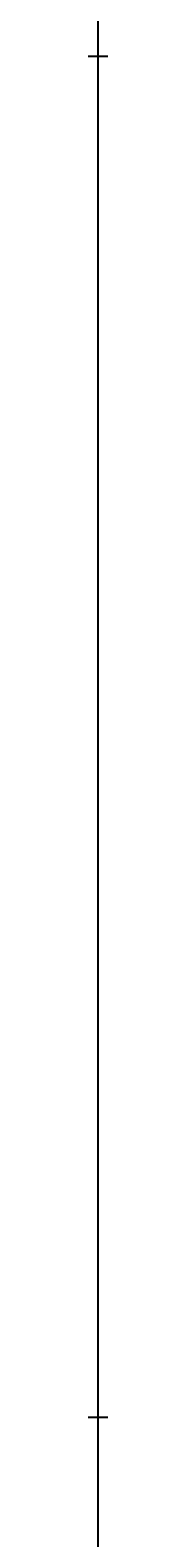
# Model space of a CAD drawing. Units: inches. Extents: x 35362 to 73946, y 43607 to 67532.
# Tile 36 of 134: x 48373 to 48373, y 46091 to 46564. Entities that reach past the tile are written whole.
import ezdxf

# ---------------------------------------------------------------- set-up
doc = ezdxf.new("R2010")
doc.units = ezdxf.units.IN
doc.header["$MEASUREMENT"] = 0
doc.layers.add('A-ANNO-DIMS', color=2, linetype='Continuous', lineweight=18)
doc.styles.get("Standard").update_dxf_attribs({"font": 'arial.ttf'})
doc.dimstyles.get("Standard").update_dxf_attribs({"dimtxt": 0.18, "dimasz": 0.18, "dimexe": 0.18, "dimexo": 0.0625, "dimgap": 0.09, "dimtad": 0, "dimtih": 1, "dimtoh": 1, "dimdec": 4, "dimzin": 0, "dimdsep": 46, "dimtxsty": 'Standard', "dimcen": 0.09, "dimadec": 0, "dimazin": 0, "dimtfac": 1, "dimtdec": 4, "dimtofl": 0, "dimtmove": 0, "dimatfit": 3, "dimfxl": 1, "dimtolj": 1, "dimtzin": 0, "dimarcsym": 0})

# ---------------------------------------------------------------- blocks, each defined once
blk = doc.blocks.new('*D5')
at = {"layer": 'A-ANNO-DIMS', "color": 0, "lineweight": -2, "transparency": 16777216}
for p, q in [((37121.95, 46919.32), (37121.95, 43606.68)), ((69871.5, 45449.83), (69871.5, 43606.68)), ((37122.13, 43606.86), (53496.29, 43606.86)), ((69871.32, 43606.86), (53497.15, 43606.86))]:
    blk.add_line(p, q, dxfattribs=at)
at = {"layer": 'A-ANNO-DIMS', "color": 0, "transparency": 16777216}
for points in [[(37122.13, 43606.89), (37122.13, 43606.83), (37121.95, 43606.86)], [(69871.32, 43606.89), (69871.32, 43606.83), (69871.5, 43606.86)]]:
    blk.add_solid(points, dxfattribs=at)
at = {"layer": 'Defpoints', "color": 0, "transparency": 16777216}
for p in [(37121.95, 46919.38), (69871.5, 45449.89), (69871.5, 43606.86)]:
    blk.add_point(p, dxfattribs=at)
at = {"layer": 'A-ANNO-DIMS', "color": 0, "transparency": 16777216, "insert": (53496.72, 43606.86), "char_height": 0.18, "attachment_point": 5}
blk.add_mtext('\\A1;32750', dxfattribs=at)
blk = doc.blocks.new('*D11')
at = {"layer": 'A-ANNO-DIMS', "color": 0, "lineweight": -2, "transparency": 16777216}
for p, q in [((47978.66, 56028.77), (47978.66, 43606.68)), ((53109.76, 56028.77), (53109.76, 43606.68)), ((47978.84, 43606.86), (50543.87, 43606.86)), ((53109.58, 43606.86), (50544.55, 43606.86))]:
    blk.add_line(p, q, dxfattribs=at)
at = {"layer": 'A-ANNO-DIMS', "color": 0, "transparency": 16777216}
for points in [[(47978.84, 43606.89), (47978.84, 43606.83), (47978.66, 43606.86)], [(53109.58, 43606.89), (53109.58, 43606.83), (53109.76, 43606.86)]]:
    blk.add_solid(points, dxfattribs=at)
at = {"layer": 'Defpoints', "color": 0, "transparency": 16777216}
for p in [(47978.66, 56028.84), (53109.76, 56028.84), (53109.76, 43606.86)]:
    blk.add_point(p, dxfattribs=at)
at = {"layer": 'A-ANNO-DIMS', "color": 0, "transparency": 16777216, "insert": (50544.21, 43606.86), "char_height": 0.18, "attachment_point": 5}
blk.add_mtext('\\A1;5131', dxfattribs=at)
blk = doc.blocks.new('*D13')
at = {"layer": 'A-ANNO-DIMS', "color": 0, "lineweight": -2, "transparency": 16777216}
for p, q in [((48373.49, 51694.02), (48373.49, 43606.68)), ((51029.04, 51694.02), (51029.04, 43606.68)), ((48373.67, 43606.86), (49700.8, 43606.86)), ((51028.86, 43606.86), (49701.73, 43606.86))]:
    blk.add_line(p, q, dxfattribs=at)
at = {"layer": 'A-ANNO-DIMS', "color": 0, "transparency": 16777216}
for points in [[(48373.67, 43606.89), (48373.67, 43606.83), (48373.49, 43606.86)], [(51028.86, 43606.89), (51028.86, 43606.83), (51029.04, 43606.86)]]:
    blk.add_solid(points, dxfattribs=at)
at = {"layer": 'Defpoints', "color": 0, "transparency": 16777216}
for p in [(48373.49, 51694.09), (51029.04, 51694.09), (51029.04, 43606.86)]:
    blk.add_point(p, dxfattribs=at)
at = {"layer": 'A-ANNO-DIMS', "color": 0, "transparency": 16777216, "insert": (49701.27, 43606.86), "char_height": 0.18, "attachment_point": 5}
blk.add_mtext('\\A1;2655.6', dxfattribs=at)
blk = doc.blocks.new('*D67')
at = {"layer": 'A-ANNO-DIMS', "color": 0, "lineweight": -2, "transparency": 16777216}
for p, q in [((56873.54, 53351.53), (35361.77, 53351.53)), ((35361.95, 53351.35), (35361.95, 49400.89)), ((35361.95, 45450.07), (35361.95, 49400.53)), ((53793.58, 45449.89), (35361.77, 45449.89))]:
    blk.add_line(p, q, dxfattribs=at)
at = {"layer": 'A-ANNO-DIMS', "color": 0, "transparency": 16777216}
for points in [[(35361.92, 53351.35), (35361.98, 53351.35), (35361.95, 53351.53)], [(35361.92, 45450.07), (35361.98, 45450.07), (35361.95, 45449.89)]]:
    blk.add_solid(points, dxfattribs=at)
at = {"layer": 'Defpoints', "color": 0, "transparency": 16777216}
for p in [(35361.95, 53351.53), (56873.6, 53351.53), (53793.64, 45449.89)]:
    blk.add_point(p, dxfattribs=at)
at = {"layer": 'A-ANNO-DIMS', "color": 0, "transparency": 16777216, "insert": (35361.95, 49400.71), "char_height": 0.18, "attachment_point": 5}
blk.add_mtext('\\A1;7901.6', dxfattribs=at)
blk = doc.blocks.new('*D76')
at = {"layer": 'A-ANNO-DIMS', "color": 0, "lineweight": -2, "transparency": 16777216}
for p, q in [((54052.84, 46555.29), (35361.77, 46555.29)), ((35361.95, 46555.11), (35361.95, 46342.27)), ((35361.95, 46129.06), (35361.95, 46341.9)), ((53793.58, 46128.88), (35361.77, 46128.88))]:
    blk.add_line(p, q, dxfattribs=at)
at = {"layer": 'A-ANNO-DIMS', "color": 0, "transparency": 16777216}
for points in [[(35361.92, 46555.11), (35361.98, 46555.11), (35361.95, 46555.29)], [(35361.92, 46129.06), (35361.98, 46129.06), (35361.95, 46128.88)]]:
    blk.add_solid(points, dxfattribs=at)
at = {"layer": 'Defpoints', "color": 0, "transparency": 16777216}
for p in [(35361.95, 46555.29), (54052.9, 46555.29), (53793.64, 46128.88)]:
    blk.add_point(p, dxfattribs=at)
at = {"layer": 'A-ANNO-DIMS', "color": 0, "transparency": 16777216, "insert": (35361.95, 46342.09), "char_height": 0.18, "attachment_point": 5}
blk.add_mtext('\\A1;426.4', dxfattribs=at)
blk = doc.blocks.new('*D90')
at = {"layer": 'A-ANNO-DIMS', "color": 0, "lineweight": -2, "transparency": 16777216}
for p, q in [((53707.72, 47291.29), (35361.77, 47291.29)), ((35361.95, 47291.11), (35361.95, 46710.26)), ((35361.95, 46129.06), (35361.95, 46709.9)), ((53793.58, 46128.88), (35361.77, 46128.88))]:
    blk.add_line(p, q, dxfattribs=at)
at = {"layer": 'A-ANNO-DIMS', "color": 0, "transparency": 16777216}
for points in [[(35361.92, 47291.11), (35361.98, 47291.11), (35361.95, 47291.29)], [(35361.92, 46129.06), (35361.98, 46129.06), (35361.95, 46128.88)]]:
    blk.add_solid(points, dxfattribs=at)
at = {"layer": 'Defpoints', "color": 0, "transparency": 16777216}
for p in [(53707.78, 47291.29), (35361.95, 46128.88), (53793.64, 46128.88)]:
    blk.add_point(p, dxfattribs=at)
at = {"layer": 'A-ANNO-DIMS', "color": 0, "transparency": 16777216, "insert": (35361.95, 46710.08), "char_height": 0.18, "attachment_point": 5}
blk.add_mtext('\\A1;1162.4', dxfattribs=at)

msp = doc.modelspace()

# ---------------------------------------------------------------- dimensions: what is measured, and where the dimension line sits
at = {"layer": 'A-ANNO-DIMS'}
for base, p1, p2, override, picture, middle in [((53109.76, 43606.859), (47978.665, 56028.836), (53109.76, 56028.836), {"dimdec": 0, "dimlfac": 1, "dimrnd": 0, "dimzin": 0, "dimdsep": 46, "dimlunit": 2}, '*D11', (50544.212, 43606.859)), ((51029.043, 43606.859), (48373.492, 51694.087), (51029.043, 51694.087), {"dimdec": 1, "dimlfac": 1, "dimrnd": 0, "dimzin": 0, "dimdsep": 46, "dimlunit": 2}, '*D13', (49701.267, 43606.859)), ((69871.496, 43606.859), (37121.949, 46919.381), (69871.496, 45449.894), {"dimdec": 0, "dimlfac": 1, "dimrnd": 0, "dimzin": 0, "dimdsep": 46, "dimlunit": 2}, '*D5', (53496.723, 43606.859))]:
    dim = msp.add_linear_dim(base=base, p1=p1, p2=p2, dimstyle='Standard', override=override, dxfattribs=at)
    dim.commit()
    dim.dimension.update_dxf_attribs({"geometry": picture, "text_midpoint": middle})
for base, p1, p2, picture, middle in [((35361.949, 53351.529), (53793.638, 45449.894), (56873.602, 53351.529), '*D67', (35361.949, 49400.712)), ((35361.949, 46128.878), (53707.781, 47291.285), (53793.638, 46128.878), '*D90', (35361.949, 46710.081)), ((35361.949, 46555.293), (53793.638, 46128.878), (54052.899, 46555.293), '*D76', (35361.949, 46342.086))]:
    dim = msp.add_linear_dim(base=base, p1=p1, p2=p2, angle=90, dimstyle='Standard', override={"dimdec": 1, "dimlfac": 1, "dimrnd": 0, "dimzin": 0, "dimdsep": 46, "dimlunit": 2}, dxfattribs=at)
    dim.commit()
    dim.dimension.update_dxf_attribs({"geometry": picture, "text_midpoint": middle})

doc.saveas('drawing.dxf')
